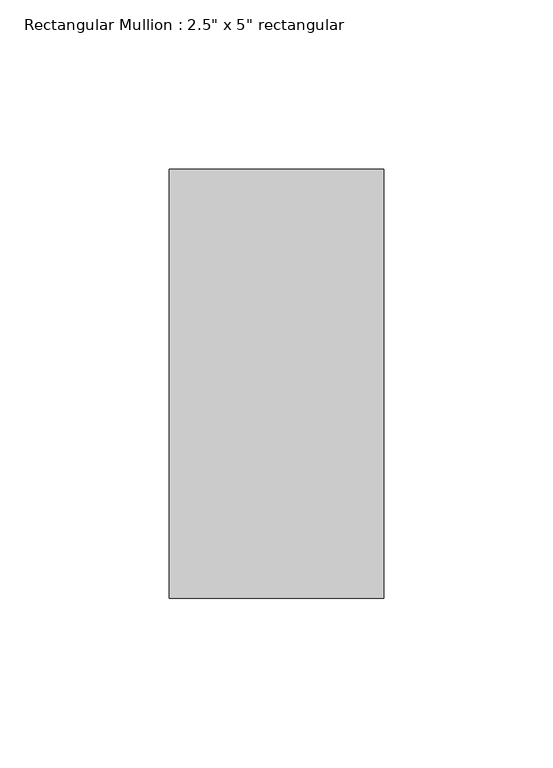
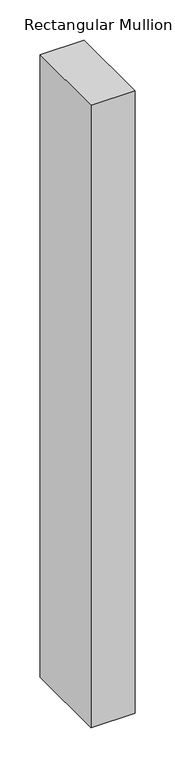
"""IFC4 building model written with IfcOpenShell, lengths in millimetres: member geometry."""

from ifc_helpers import new_model, si_unit, frame, origin, place, context, project, spatial, polyline, outline, extrude, source, transform, mapped, element, save


def member_a24dc69d(model_context):
    return source(origin(), model_context, "Body", "SweptSolid", [
        extrude(outline(polyline([(31.75, 63.5), (31.75, -63.5), (-31.75, -63.5), (-31.75, 63.5), (31.75, 63.5)])), frame((0.0, 0.0, -947.4497825), z_axis=(0.0, 0.0, 1.0), x_axis=(1.0, 0.0, 0.0)), (0.0, 0.0, 1.0), 947.4497825),
    ])


if __name__ == "__main__":
    model = new_model("IFC4")
    model_context = context("Model", 3, world=origin())
    ifc_project = project(units=[si_unit("LENGTHUNIT", "METRE", prefix="MILLI")], contexts=[model_context])
    site = spatial("IfcSite", under=ifc_project)
    building = spatial("IfcBuilding", under=site)
    placement = place(None, origin())
    member_shape = member_a24dc69d(model_context)
    element("IfcMember", 1, ObjectType="Rectangular Mullion : 2.5\" x 5\" rectangular", at=placement, inside=building, context=model_context, shape_type="MappedRepresentation", body=[
        mapped(member_shape, transform((0.0, 0.0, 0.0), x_axis=(1.0, 0.0, 0.0), y_axis=(0.0, 1.0, 0.0), z_axis=(0.0, 0.0, 1.0))),
    ])
    save(model, "model.ifc")

# Revit data of these elements
# Type "Rectangular Mullion : 2.5\" x 5\" rectangular"
#   built-in parameter 1007304 = 0.416667 (stored number, unit not read)
#   built-in parameter 1007301 = 0.104167 (stored number, unit not read)
#   built-in parameter 1007300 = 0.104167 (stored number, unit not read)
# Element 1 (IfcMember, "Rectangular Mullion : 2.5\" x 5\" rectangular")
#   Materials on its faces: "BLACK COLOUR"
# Materials
#   "BLACK COLOUR": class "Generic", colour RGB 120 120 120, transparency 0, Cost = 0
